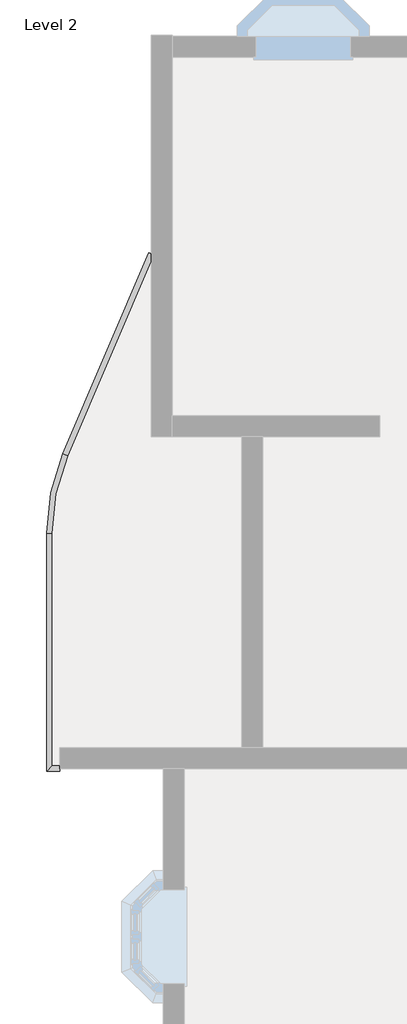
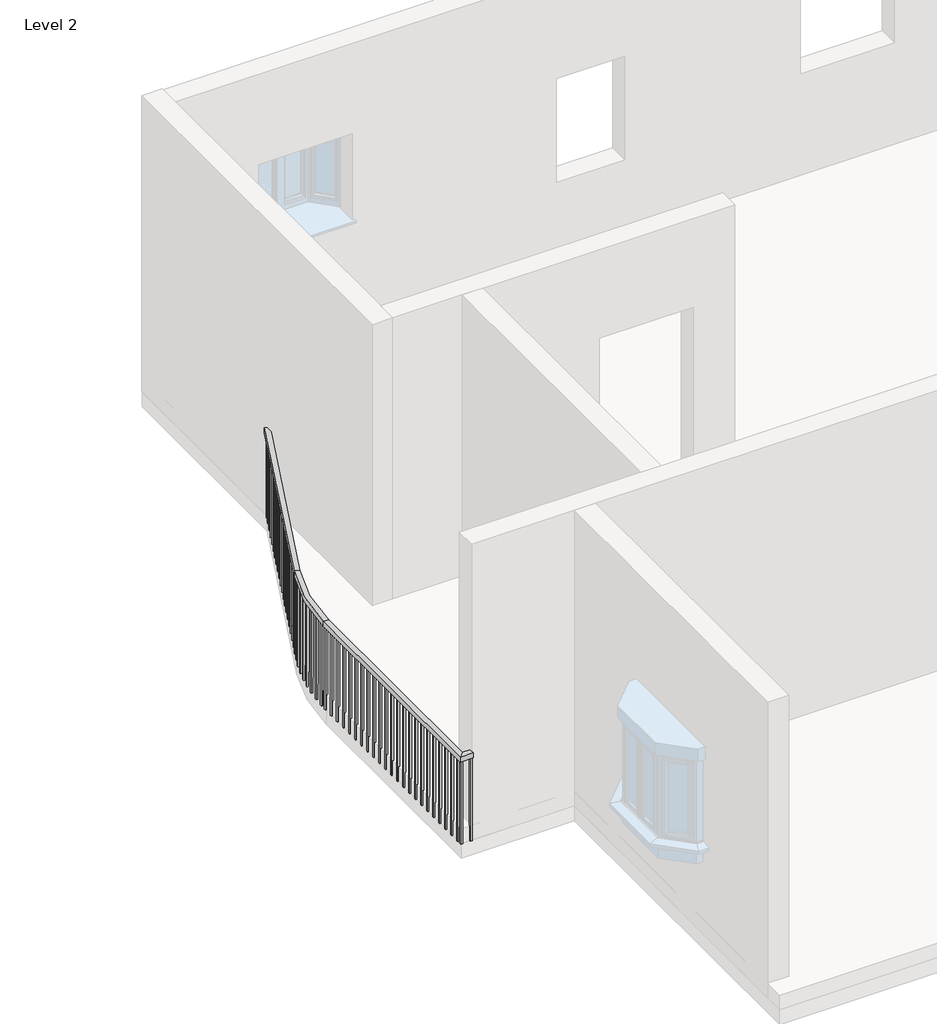
# One storey, part 7 of 14: 1 railing.
"""IFC4 building model written with IfcOpenShell, lengths in millimetres."""

from ifc_helpers import new_model, si_unit, frame, origin, place, context, project, spatial, polyline, circle_curve, outline, extrude, element, save
from ifc_brep_helpers import plane_surface, cylinder_surface, revolved_surface, advanced_brep

model = new_model("IFC4")

# Units and contexts
model_context = context("Model", 3, world=origin())
ifc_project = project(units=[si_unit("LENGTHUNIT", "METRE", prefix="MILLI")], contexts=[model_context])

# Site, building, storey
site = spatial("IfcSite", under=ifc_project)
building = spatial("IfcBuilding", under=site)
storey = spatial("IfcBuildingStorey", under=building, Name="Level 2", Elevation=3048.0)

# Railing
placement = place(None, origin())
element("IfcRailing", 1, ObjectType="Handrail - Rectangular", at=placement, inside=storey, context=model_context, shape_type="SolidModel", body=[
    advanced_brep(
    [(-12381.4379579, -2441.2590879, 3962.4), (-12381.4379579, -2441.2590879, 3911.6), (-12428.1364721, -2421.2618688, 3911.6), (-12428.1364721, -2421.2618688, 3962.4), (-13216.1814979, -4390.5942894, 3962.4), (-13216.1814979, -4390.5942894, 3911.6), (-13262.8800121, -4370.5970703, 3911.6), (-13262.8800121, -4370.5970703, 3962.4), (-13369.987215, -5140.4900045, 3911.6), (-13369.987215, -5140.4900045, 3962.4), (-13420.787215, -5140.4900045, 3911.6), (-13420.787215, -5140.4900045, 3962.4), (-13369.987215, -7396.5416506, 3962.4), (-13369.987215, -7396.5416506, 3911.6), (-13420.787215, -7447.3416506, 3911.6), (-13420.787215, -7447.3416506, 3962.4), (-13293.787215, -7396.5416506, 3962.4), (-13293.787215, -7447.3416506, 3962.4), (-13293.787215, -7447.3416506, 3911.6), (-13293.787215, -7396.5416506, 3911.6)],
    [
        (0, 1),
        (1, 2),
        (2, 3),
        (3, 0),
        (0, 4),
        (4, 5),
        (5, 1),
        (5, 6),
        (6, 2),
        (6, 7),
        (7, 3),
        (7, 4),
        (8, 5, circle_curve(frame((-11464.987215, -5140.4900045, 3911.6), z_axis=(0.0, 0.0, -1.0), x_axis=(-0.9192620907623802, 0.39364604467360964, 0.0)), 1905.0)),
        (4, 9, circle_curve(frame((-11464.987215, -5140.4900045, 3962.4), z_axis=(0.0, 0.0, 1.0), x_axis=(-0.9192620907623802, 0.39364604467360964, 0.0)), 1905.0)),
        (9, 8),
        (10, 6, circle_curve(frame((-11464.987215, -5140.4900045, 3911.6), z_axis=(0.0, 0.0, -1.0), x_axis=(-0.9192620907623802, 0.39364604467360964, 0.0)), 1955.8)),
        (8, 10),
        (11, 7, circle_curve(frame((-11464.987215, -5140.4900045, 3962.4), z_axis=(0.0, 0.0, -1.0), x_axis=(-0.9192620907623802, 0.39364604467360964, 0.0)), 1955.8)),
        (10, 11),
        (11, 9),
        (9, 12),
        (12, 13),
        (13, 8),
        (13, 14),
        (14, 10),
        (14, 15),
        (15, 11),
        (15, 12),
        (16, 17),
        (17, 18),
        (18, 19),
        (19, 16),
        (12, 16),
        (19, 13),
        (18, 14),
        (17, 15),
    ],
    [
        plane_surface(frame((-12404.787215, -2431.2604783, 3962.4), z_axis=(0.39364604467361003, 0.9192620907623801, 0.0), x_axis=(0.9192620907623801, -0.39364604467361003, 0.0))),
        plane_surface(frame((-12381.4379579, -2441.2590879, 3962.4), z_axis=(0.9192620907623801, -0.3936460446736101, 0.0), x_axis=(-0.3936460446736101, -0.9192620907623801, 0.0))),
        plane_surface(frame((-12381.4379579, -2441.2590879, 3911.6), z_axis=(0.0, 0.0, -1.0000000000000002), x_axis=(-0.3936460446736101, -0.9192620907623801, 0.0))),
        plane_surface(frame((-12428.1364721, -2421.2618688, 3911.6), z_axis=(-0.9192620907623801, 0.39364604467361, 0.0), x_axis=(-0.39364604467361, -0.9192620907623801, 0.0))),
        plane_surface(frame((-12428.1364721, -2421.2618688, 3962.4), z_axis=(0.0, 0.0, 1.0), x_axis=(-0.39364604467361, -0.9192620907623801, 0.0))),
        revolved_surface(polyline([(-13216.181497902333, -4390.594289396774, 3962.4), (-13216.181497902333, -4390.594289396774, 3911.6)]), (-11464.987215, -5140.4900045, 3962.4), (0.0, 0.0, 1.0)),
        plane_surface(frame((-11464.987215, -5140.4900045, 3911.6), z_axis=(0.0, 0.0, -1.0), x_axis=(-0.9192620907623802, 0.39364604467360964, 0.0))),
        cylinder_surface(frame((-11464.987215, -5140.4900045, 3962.4), z_axis=(0.0, 0.0, 1.0), x_axis=(-0.9192620907623802, 0.39364604467360964, 0.0)), 1955.8),
        plane_surface(frame((-11464.987215, -5140.4900045, 3962.4), z_axis=(0.0, 0.0, 1.0), x_axis=(-0.9192620907623802, 0.39364604467360964, 0.0))),
        plane_surface(frame((-13369.987215, -5140.4900045, 3962.4), z_axis=(1.0, 0.0, 0.0), x_axis=(0.0, -1.0, 0.0))),
        plane_surface(frame((-13369.987215, -5140.4900045, 3911.6), z_axis=(0.0, 0.0, -1.0), x_axis=(0.0, -1.0, 0.0))),
        plane_surface(frame((-13420.787215, -5140.4900045, 3911.6), z_axis=(-1.0, 0.0, 0.0), x_axis=(0.0, -1.0, 0.0))),
        plane_surface(frame((-13420.787215, -5140.4900045, 3962.4), z_axis=(0.0, 0.0, 1.0), x_axis=(0.0, -1.0, 0.0))),
        plane_surface(frame((-13293.787215, -7421.9416506, 3962.4), z_axis=(1.0, 0.0, 0.0), x_axis=(0.0, 1.0, 0.0))),
        plane_surface(frame((-13369.987215, -7396.5416506, 3962.4), z_axis=(0.0, 1.0, 0.0), x_axis=(1.0, 0.0, 0.0))),
        plane_surface(frame((-13369.987215, -7396.5416506, 3911.6), z_axis=(0.0, 0.0, -1.0), x_axis=(1.0, 0.0, 0.0))),
        plane_surface(frame((-13420.787215, -7447.3416506, 3911.6), z_axis=(0.0, -1.0, 0.0), x_axis=(1.0, 0.0, 0.0))),
        plane_surface(frame((-13420.787215, -7447.3416506, 3962.4), z_axis=(0.0, 0.0, 1.0), x_axis=(1.0, 0.0, 0.0))),
    ],
    [
        (0, [[1, 2, 3, 4]]),
        (1, [[-1, 5, 6, 7]]),
        (2, [[-2, -7, 8, 9]]),
        (3, [[-3, -9, 10, 11]]),
        (4, [[-4, -11, 12, -5]]),
        (5, [[13, -6, 14, 15]]),
        (6, [[16, -8, -13, 17]]),
        (7, [[18, -10, -16, 19]]),
        (8, [[-14, -12, -18, 20]]),
        (9, [[-15, 21, 22, 23]]),
        (10, [[-17, -23, 24, 25]]),
        (11, [[-19, -25, 26, 27]]),
        (12, [[-20, -27, 28, -21]]),
        (13, [[29, 30, 31, 32]]),
        (14, [[-22, 33, -32, 34]]),
        (15, [[-24, -34, -31, 35]]),
        (16, [[-26, -35, -30, 36]]),
        (17, [[-28, -36, -29, -33]]),
    ],
),
    extrude(outline(polyline([(-13404.912215, -7366.1650045), (-13385.862215, -7366.1650045), (-13385.862215, -7385.2150045), (-13404.912215, -7385.2150045), (-13404.912215, -7366.1650045)])), frame((0.0, 0.0, 3048.0), z_axis=(0.0, 0.0, 1.0), x_axis=(1.0, 0.0, 0.0)), (0.0, 0.0, 1.0), 863.6),
    extrude(outline(polyline([(-13404.912215, -7264.5650045), (-13385.862215, -7264.5650045), (-13385.862215, -7283.6150045), (-13404.912215, -7283.6150045), (-13404.912215, -7264.5650045)])), frame((0.0, 0.0, 3048.0), z_axis=(0.0, 0.0, 1.0), x_axis=(1.0, 0.0, 0.0)), (0.0, 0.0, 1.0), 863.6),
    extrude(outline(polyline([(-13404.912215, -7162.9650045), (-13385.862215, -7162.9650045), (-13385.862215, -7182.0150045), (-13404.912215, -7182.0150045), (-13404.912215, -7162.9650045)])), frame((0.0, 0.0, 3048.0), z_axis=(0.0, 0.0, 1.0), x_axis=(1.0, 0.0, 0.0)), (0.0, 0.0, 1.0), 863.6),
    extrude(outline(polyline([(-13404.912215, -7061.3650045), (-13385.862215, -7061.3650045), (-13385.862215, -7080.4150045), (-13404.912215, -7080.4150045), (-13404.912215, -7061.3650045)])), frame((0.0, 0.0, 3048.0), z_axis=(0.0, 0.0, 1.0), x_axis=(1.0, 0.0, 0.0)), (0.0, 0.0, 1.0), 863.6),
    extrude(outline(polyline([(-13404.912215, -6959.7650045), (-13385.862215, -6959.7650045), (-13385.862215, -6978.8150045), (-13404.912215, -6978.8150045), (-13404.912215, -6959.7650045)])), frame((0.0, 0.0, 3048.0), z_axis=(0.0, 0.0, 1.0), x_axis=(1.0, 0.0, 0.0)), (0.0, 0.0, 1.0), 863.6),
    extrude(outline(polyline([(-13404.912215, -6858.1650045), (-13385.862215, -6858.1650045), (-13385.862215, -6877.2150045), (-13404.912215, -6877.2150045), (-13404.912215, -6858.1650045)])), frame((0.0, 0.0, 3048.0), z_axis=(0.0, 0.0, 1.0), x_axis=(1.0, 0.0, 0.0)), (0.0, 0.0, 1.0), 863.6),
    extrude(outline(polyline([(-13404.912215, -6756.5650045), (-13385.862215, -6756.5650045), (-13385.862215, -6775.6150045), (-13404.912215, -6775.6150045), (-13404.912215, -6756.5650045)])), frame((0.0, 0.0, 3048.0), z_axis=(0.0, 0.0, 1.0), x_axis=(1.0, 0.0, 0.0)), (0.0, 0.0, 1.0), 863.6),
    extrude(outline(polyline([(-13404.912215, -6654.9650045), (-13385.862215, -6654.9650045), (-13385.862215, -6674.0150045), (-13404.912215, -6674.0150045), (-13404.912215, -6654.9650045)])), frame((0.0, 0.0, 3048.0), z_axis=(0.0, 0.0, 1.0), x_axis=(1.0, 0.0, 0.0)), (0.0, 0.0, 1.0), 863.6),
    extrude(outline(polyline([(-13404.912215, -6553.3650045), (-13385.862215, -6553.3650045), (-13385.862215, -6572.4150045), (-13404.912215, -6572.4150045), (-13404.912215, -6553.3650045)])), frame((0.0, 0.0, 3048.0), z_axis=(0.0, 0.0, 1.0), x_axis=(1.0, 0.0, 0.0)), (0.0, 0.0, 1.0), 863.6),
    extrude(outline(polyline([(-13404.912215, -6451.7650045), (-13385.862215, -6451.7650045), (-13385.862215, -6470.8150045), (-13404.912215, -6470.8150045), (-13404.912215, -6451.7650045)])), frame((0.0, 0.0, 3048.0), z_axis=(0.0, 0.0, 1.0), x_axis=(1.0, 0.0, 0.0)), (0.0, 0.0, 1.0), 863.6),
    extrude(outline(polyline([(-13404.912215, -6350.1650045), (-13385.862215, -6350.1650045), (-13385.862215, -6369.2150045), (-13404.912215, -6369.2150045), (-13404.912215, -6350.1650045)])), frame((0.0, 0.0, 3048.0), z_axis=(0.0, 0.0, 1.0), x_axis=(1.0, 0.0, 0.0)), (0.0, 0.0, 1.0), 863.6),
    extrude(outline(polyline([(-13404.912215, -6248.5650045), (-13385.862215, -6248.5650045), (-13385.862215, -6267.6150045), (-13404.912215, -6267.6150045), (-13404.912215, -6248.5650045)])), frame((0.0, 0.0, 3048.0), z_axis=(0.0, 0.0, 1.0), x_axis=(1.0, 0.0, 0.0)), (0.0, 0.0, 1.0), 863.6),
    extrude(outline(polyline([(-13404.912215, -6146.9650045), (-13385.862215, -6146.9650045), (-13385.862215, -6166.0150045), (-13404.912215, -6166.0150045), (-13404.912215, -6146.9650045)])), frame((0.0, 0.0, 3048.0), z_axis=(0.0, 0.0, 1.0), x_axis=(1.0, 0.0, 0.0)), (0.0, 0.0, 1.0), 863.6),
    extrude(outline(polyline([(-13404.912215, -6045.3650045), (-13385.862215, -6045.3650045), (-13385.862215, -6064.4150045), (-13404.912215, -6064.4150045), (-13404.912215, -6045.3650045)])), frame((0.0, 0.0, 3048.0), z_axis=(0.0, 0.0, 1.0), x_axis=(1.0, 0.0, 0.0)), (0.0, 0.0, 1.0), 863.6),
    extrude(outline(polyline([(-13404.912215, -5943.7650045), (-13385.862215, -5943.7650045), (-13385.862215, -5962.8150045), (-13404.912215, -5962.8150045), (-13404.912215, -5943.7650045)])), frame((0.0, 0.0, 3048.0), z_axis=(0.0, 0.0, 1.0), x_axis=(1.0, 0.0, 0.0)), (0.0, 0.0, 1.0), 863.6),
    extrude(outline(polyline([(-13404.912215, -5842.1650045), (-13385.862215, -5842.1650045), (-13385.862215, -5861.2150045), (-13404.912215, -5861.2150045), (-13404.912215, -5842.1650045)])), frame((0.0, 0.0, 3048.0), z_axis=(0.0, 0.0, 1.0), x_axis=(1.0, 0.0, 0.0)), (0.0, 0.0, 1.0), 863.6),
    extrude(outline(polyline([(-13404.912215, -5740.5650045), (-13385.862215, -5740.5650045), (-13385.862215, -5759.6150045), (-13404.912215, -5759.6150045), (-13404.912215, -5740.5650045)])), frame((0.0, 0.0, 3048.0), z_axis=(0.0, 0.0, 1.0), x_axis=(1.0, 0.0, 0.0)), (0.0, 0.0, 1.0), 863.6),
    extrude(outline(polyline([(-13404.912215, -5638.9650045), (-13385.862215, -5638.9650045), (-13385.862215, -5658.0150045), (-13404.912215, -5658.0150045), (-13404.912215, -5638.9650045)])), frame((0.0, 0.0, 3048.0), z_axis=(0.0, 0.0, 1.0), x_axis=(1.0, 0.0, 0.0)), (0.0, 0.0, 1.0), 863.6),
    extrude(outline(polyline([(-13404.912215, -5537.3650045), (-13385.862215, -5537.3650045), (-13385.862215, -5556.4150045), (-13404.912215, -5556.4150045), (-13404.912215, -5537.3650045)])), frame((0.0, 0.0, 3048.0), z_axis=(0.0, 0.0, 1.0), x_axis=(1.0, 0.0, 0.0)), (0.0, 0.0, 1.0), 863.6),
    extrude(outline(polyline([(-13404.912215, -5435.7650045), (-13385.862215, -5435.7650045), (-13385.862215, -5454.8150045), (-13404.912215, -5454.8150045), (-13404.912215, -5435.7650045)])), frame((0.0, 0.0, 3048.0), z_axis=(0.0, 0.0, 1.0), x_axis=(1.0, 0.0, 0.0)), (0.0, 0.0, 1.0), 863.6),
    extrude(outline(polyline([(-13404.912215, -5334.1650045), (-13385.862215, -5334.1650045), (-13385.862215, -5353.2150045), (-13404.912215, -5353.2150045), (-13404.912215, -5334.1650045)])), frame((0.0, 0.0, 3048.0), z_axis=(0.0, 0.0, 1.0), x_axis=(1.0, 0.0, 0.0)), (0.0, 0.0, 1.0), 863.6),
    extrude(outline(polyline([(-13404.912215, -5232.5650045), (-13385.862215, -5232.5650045), (-13385.862215, -5251.6150045), (-13404.912215, -5251.6150045), (-13404.912215, -5232.5650045)])), frame((0.0, 0.0, 3048.0), z_axis=(0.0, 0.0, 1.0), x_axis=(1.0, 0.0, 0.0)), (0.0, 0.0, 1.0), 863.6),
    extrude(outline(polyline([(-13403.2986616, -5060.8127369), (-13384.2611239, -5061.5016911), (-13384.9500781, -5080.5392288), (-13403.9876158, -5079.8502746), (-13403.2986616, -5060.8127369)])), frame((0.0, 0.0, 3048.0), z_axis=(0.0, 0.0, 1.0), x_axis=(1.0, 0.0, 0.0)), (0.0, 0.0, 1.0), 863.6),
    extrude(outline(polyline([(-13396.4230348, -4958.9537683), (-13377.4481028, -4960.6432816), (-13379.1376161, -4979.6182136), (-13398.1125481, -4977.9287003), (-13396.4230348, -4958.9537683)])), frame((0.0, 0.0, 3048.0), z_axis=(0.0, 0.0, 1.0), x_axis=(1.0, 0.0, 0.0)), (0.0, 0.0, 1.0), 863.6),
    extrude(outline(polyline([(-13384.1984052, -4857.5975541), (-13365.3386289, -4860.2829475), (-13368.0240223, -4879.1427238), (-13386.8837986, -4876.4573304), (-13384.1984052, -4857.5975541)])), frame((0.0, 0.0, 3048.0), z_axis=(0.0, 0.0, 1.0), x_axis=(1.0, 0.0, 0.0)), (0.0, 0.0, 1.0), 863.6),
    extrude(outline(polyline([(-13366.6586282, -4757.0247946), (-13347.9662387, -4760.698631), (-13351.6400752, -4779.3910205), (-13370.3324647, -4775.7171841), (-13366.6586282, -4757.0247946)])), frame((0.0, 0.0, 3048.0), z_axis=(0.0, 0.0, 1.0), x_axis=(1.0, 0.0, 0.0)), (0.0, 0.0, 1.0), 863.6),
    extrude(outline(polyline([(-13343.8522793, -4657.5140204), (-13325.3790441, -4662.1661254), (-13330.0311492, -4680.6393606), (-13348.5043844, -4675.9872556), (-13343.8522793, -4657.5140204)])), frame((0.0, 0.0, 3048.0), z_axis=(0.0, 0.0, 1.0), x_axis=(1.0, 0.0, 0.0)), (0.0, 0.0, 1.0), 863.6),
    extrude(outline(polyline([(-13315.8425193, -4559.340821), (-13297.6395991, -4564.9583109), (-13303.257089, -4583.1612312), (-13321.4600093, -4577.5437413), (-13315.8425193, -4559.340821)])), frame((0.0, 0.0, 3048.0), z_axis=(0.0, 0.0, 1.0), x_axis=(1.0, 0.0, 0.0)), (0.0, 0.0, 1.0), 863.6),
    extrude(outline(polyline([(-13282.7069198, -4462.7770815), (-13264.8247264, -4469.344399), (-13271.3920438, -4487.2265924), (-13289.2742372, -4480.659275), (-13282.7069198, -4462.7770815)])), frame((0.0, 0.0, 3048.0), z_axis=(0.0, 0.0, 1.0), x_axis=(1.0, 0.0, 0.0)), (0.0, 0.0, 1.0), 863.6),
    extrude(outline(polyline([(-13209.6824706, -4286.6955968), (-13192.1705278, -4294.1945539), (-13199.6694849, -4311.7064967), (-13217.1814277, -4304.2075396), (-13209.6824706, -4286.6955968)])), frame((0.0, 0.0, 3048.0), z_axis=(0.0, 0.0, 1.0), x_axis=(1.0, 0.0, 0.0)), (0.0, 0.0, 1.0), 863.6),
    extrude(outline(polyline([(-13169.6880325, -4193.2985683), (-13152.1760896, -4200.7975255), (-13159.6750468, -4218.3094683), (-13177.1869896, -4210.8105112), (-13169.6880325, -4193.2985683)])), frame((0.0, 0.0, 3048.0), z_axis=(0.0, 0.0, 1.0), x_axis=(1.0, 0.0, 0.0)), (0.0, 0.0, 1.0), 863.6),
    extrude(outline(polyline([(-13129.6935943, -4099.9015399), (-13112.1816515, -4107.4004971), (-13119.6806086, -4124.9124399), (-13137.1925515, -4117.4134827), (-13129.6935943, -4099.9015399)])), frame((0.0, 0.0, 3048.0), z_axis=(0.0, 0.0, 1.0), x_axis=(1.0, 0.0, 0.0)), (0.0, 0.0, 1.0), 863.6),
    extrude(outline(polyline([(-13089.6991562, -4006.5045115), (-13072.1872133, -4014.0034686), (-13079.6861705, -4031.5154115), (-13097.1981133, -4024.0164543), (-13089.6991562, -4006.5045115)])), frame((0.0, 0.0, 3048.0), z_axis=(0.0, 0.0, 1.0), x_axis=(1.0, 0.0, 0.0)), (0.0, 0.0, 1.0), 863.6),
    extrude(outline(polyline([(-13049.704718, -3913.1074831), (-13032.1927752, -3920.6064402), (-13039.6917324, -3938.1183831), (-13057.2036752, -3930.6194259), (-13049.704718, -3913.1074831)])), frame((0.0, 0.0, 3048.0), z_axis=(0.0, 0.0, 1.0), x_axis=(1.0, 0.0, 0.0)), (0.0, 0.0, 1.0), 863.6),
    extrude(outline(polyline([(-13009.7102799, -3819.7104546), (-12992.1983371, -3827.2094118), (-12999.6972942, -3844.7213546), (-13017.209237, -3837.2223975), (-13009.7102799, -3819.7104546)])), frame((0.0, 0.0, 3048.0), z_axis=(0.0, 0.0, 1.0), x_axis=(1.0, 0.0, 0.0)), (0.0, 0.0, 1.0), 863.6),
    extrude(outline(polyline([(-12969.7158418, -3726.3134262), (-12952.2038989, -3733.8123834), (-12959.7028561, -3751.3243262), (-12977.2147989, -3743.8253691), (-12969.7158418, -3726.3134262)])), frame((0.0, 0.0, 3048.0), z_axis=(0.0, 0.0, 1.0), x_axis=(1.0, 0.0, 0.0)), (0.0, 0.0, 1.0), 863.6),
    extrude(outline(polyline([(-12929.7214036, -3632.9163978), (-12912.2094608, -3640.415355), (-12919.7084179, -3657.9272978), (-12937.2203608, -3650.4283406), (-12929.7214036, -3632.9163978)])), frame((0.0, 0.0, 3048.0), z_axis=(0.0, 0.0, 1.0), x_axis=(1.0, 0.0, 0.0)), (0.0, 0.0, 1.0), 863.6),
    extrude(outline(polyline([(-12889.7269655, -3539.5193694), (-12872.2150227, -3547.0183265), (-12879.7139798, -3564.5302694), (-12897.2259226, -3557.0313122), (-12889.7269655, -3539.5193694)])), frame((0.0, 0.0, 3048.0), z_axis=(0.0, 0.0, 1.0), x_axis=(1.0, 0.0, 0.0)), (0.0, 0.0, 1.0), 863.6),
    extrude(outline(polyline([(-12849.7325273, -3446.122341), (-12832.2205845, -3453.6212981), (-12839.7195417, -3471.1332409), (-12857.2314845, -3463.6342838), (-12849.7325273, -3446.122341)])), frame((0.0, 0.0, 3048.0), z_axis=(0.0, 0.0, 1.0), x_axis=(1.0, 0.0, 0.0)), (0.0, 0.0, 1.0), 863.6),
    extrude(outline(polyline([(-12809.7380892, -3352.7253125), (-12792.2261464, -3360.2242697), (-12799.7251035, -3377.7362125), (-12817.2370464, -3370.2372554), (-12809.7380892, -3352.7253125)])), frame((0.0, 0.0, 3048.0), z_axis=(0.0, 0.0, 1.0), x_axis=(1.0, 0.0, 0.0)), (0.0, 0.0, 1.0), 863.6),
    extrude(outline(polyline([(-12769.7436511, -3259.3282841), (-12752.2317082, -3266.8272413), (-12759.7306654, -3284.3391841), (-12777.2426082, -3276.8402269), (-12769.7436511, -3259.3282841)])), frame((0.0, 0.0, 3048.0), z_axis=(0.0, 0.0, 1.0), x_axis=(1.0, 0.0, 0.0)), (0.0, 0.0, 1.0), 863.6),
    extrude(outline(polyline([(-12729.7492129, -3165.9312557), (-12712.2372701, -3173.4302129), (-12719.7362272, -3190.9421557), (-12737.2481701, -3183.4431985), (-12729.7492129, -3165.9312557)])), frame((0.0, 0.0, 3048.0), z_axis=(0.0, 0.0, 1.0), x_axis=(1.0, 0.0, 0.0)), (0.0, 0.0, 1.0), 863.6),
    extrude(outline(polyline([(-12689.7547748, -3072.5342273), (-12672.242832, -3080.0331844), (-12679.7417891, -3097.5451273), (-12697.2537319, -3090.0461701), (-12689.7547748, -3072.5342273)])), frame((0.0, 0.0, 3048.0), z_axis=(0.0, 0.0, 1.0), x_axis=(1.0, 0.0, 0.0)), (0.0, 0.0, 1.0), 863.6),
    extrude(outline(polyline([(-12649.7603366, -2979.1371989), (-12632.2483938, -2986.636156), (-12639.747351, -3004.1480988), (-12657.2592938, -2996.6491417), (-12649.7603366, -2979.1371989)])), frame((0.0, 0.0, 3048.0), z_axis=(0.0, 0.0, 1.0), x_axis=(1.0, 0.0, 0.0)), (0.0, 0.0, 1.0), 863.6),
    extrude(outline(polyline([(-12609.7658985, -2885.7401704), (-12592.2539557, -2893.2391276), (-12599.7529128, -2910.7510704), (-12617.2648557, -2903.2521133), (-12609.7658985, -2885.7401704)])), frame((0.0, 0.0, 3048.0), z_axis=(0.0, 0.0, 1.0), x_axis=(1.0, 0.0, 0.0)), (0.0, 0.0, 1.0), 863.6),
    extrude(outline(polyline([(-12569.7714604, -2792.343142), (-12552.2595175, -2799.8420992), (-12559.7584747, -2817.354042), (-12577.2704175, -2809.8550848), (-12569.7714604, -2792.343142)])), frame((0.0, 0.0, 3048.0), z_axis=(0.0, 0.0, 1.0), x_axis=(1.0, 0.0, 0.0)), (0.0, 0.0, 1.0), 863.6),
    extrude(outline(polyline([(-12529.7770222, -2698.9461136), (-12512.2650794, -2706.4450707), (-12519.7640366, -2723.9570136), (-12537.2759794, -2716.4580564), (-12529.7770222, -2698.9461136)])), frame((0.0, 0.0, 3048.0), z_axis=(0.0, 0.0, 1.0), x_axis=(1.0, 0.0, 0.0)), (0.0, 0.0, 1.0), 863.6),
    extrude(outline(polyline([(-12489.7825841, -2605.5490852), (-12472.2706413, -2613.0480423), (-12479.7695984, -2630.5599852), (-12497.2815412, -2623.061028), (-12489.7825841, -2605.5490852)])), frame((0.0, 0.0, 3048.0), z_axis=(0.0, 0.0, 1.0), x_axis=(1.0, 0.0, 0.0)), (0.0, 0.0, 1.0), 863.6),
    extrude(outline(polyline([(-12449.788146, -2512.1520567), (-12432.2762031, -2519.6510139), (-12439.7751603, -2537.1629567), (-12457.2871031, -2529.6639996), (-12449.788146, -2512.1520567)])), frame((0.0, 0.0, 3048.0), z_axis=(0.0, 0.0, 1.0), x_axis=(1.0, 0.0, 0.0)), (0.0, 0.0, 1.0), 863.6),
    extrude(outline(polyline([(-13404.912215, -7412.4166506), (-13385.862215, -7412.4166506), (-13385.862215, -7431.4666506), (-13404.912215, -7431.4666506), (-13404.912215, -7412.4166506)])), frame((0.0, 0.0, 3048.0), z_axis=(0.0, 0.0, 1.0), x_axis=(1.0, 0.0, 0.0)), (0.0, 0.0, 1.0), 863.6),
    extrude(outline(polyline([(-13404.912215, -5130.9650045), (-13385.862215, -5130.9650045), (-13385.862215, -5150.0150045), (-13404.912215, -5150.0150045), (-13404.912215, -5130.9650045)])), frame((0.0, 0.0, 3048.0), z_axis=(0.0, 0.0, 1.0), x_axis=(1.0, 0.0, 0.0)), (0.0, 0.0, 1.0), 863.6),
    extrude(outline(polyline([(-13244.5372478, -4368.0902299), (-13227.025305, -4375.589187), (-13234.5242621, -4393.1011299), (-13252.036205, -4385.6021727), (-13244.5372478, -4368.0902299)])), frame((0.0, 0.0, 3048.0), z_axis=(0.0, 0.0, 1.0), x_axis=(1.0, 0.0, 0.0)), (0.0, 0.0, 1.0), 863.6),
    extrude(outline(polyline([(-13312.837215, -7431.4666506), (-13312.837215, -7412.4166506), (-13293.787215, -7412.4166506), (-13293.787215, -7431.4666506), (-13312.837215, -7431.4666506)])), frame((0.0, 0.0, 3048.0), z_axis=(0.0, 0.0, 1.0), x_axis=(1.0, 0.0, 0.0)), (0.0, 0.0, 1.0), 863.6),
    extrude(outline(polyline([(-12413.5431864, -2427.5109997), (-12396.0312436, -2435.0099569), (-12403.5302007, -2452.5218997), (-12421.0421435, -2445.0229426), (-12413.5431864, -2427.5109997)])), frame((0.0, 0.0, 3048.0), z_axis=(0.0, 0.0, 1.0), x_axis=(1.0, 0.0, 0.0)), (0.0, 0.0, 1.0), 863.6),
])

save(model, "model.ifc")

# Revit data of these elements
# Type "Handrail - Rectangular"
#   Assembly Code = "C2010400"
#   built-in parameter 1008612 = 0.0416667 (stored number, unit not read)
#   built-in parameter 1008611 = 0.0416667 (stored number, unit not read)
#   built-in parameter 1008609 = 0.333333 (stored number, unit not read)
#   built-in parameter 1008604 = 0.166667 (stored number, unit not read)
#   built-in parameter 1008603 = 0.166667 (stored number, unit not read)
#   Railing Height = 3' - 0"
#   built-in parameter 1008630 = 2
#   built-in parameter 1008610 = 2
#   built-in parameter 1008618 = Baluster - Square : 3/4"
# Element 1 (IfcRailing, "Handrail - Rectangular")
#   Phase Created = New Construction
